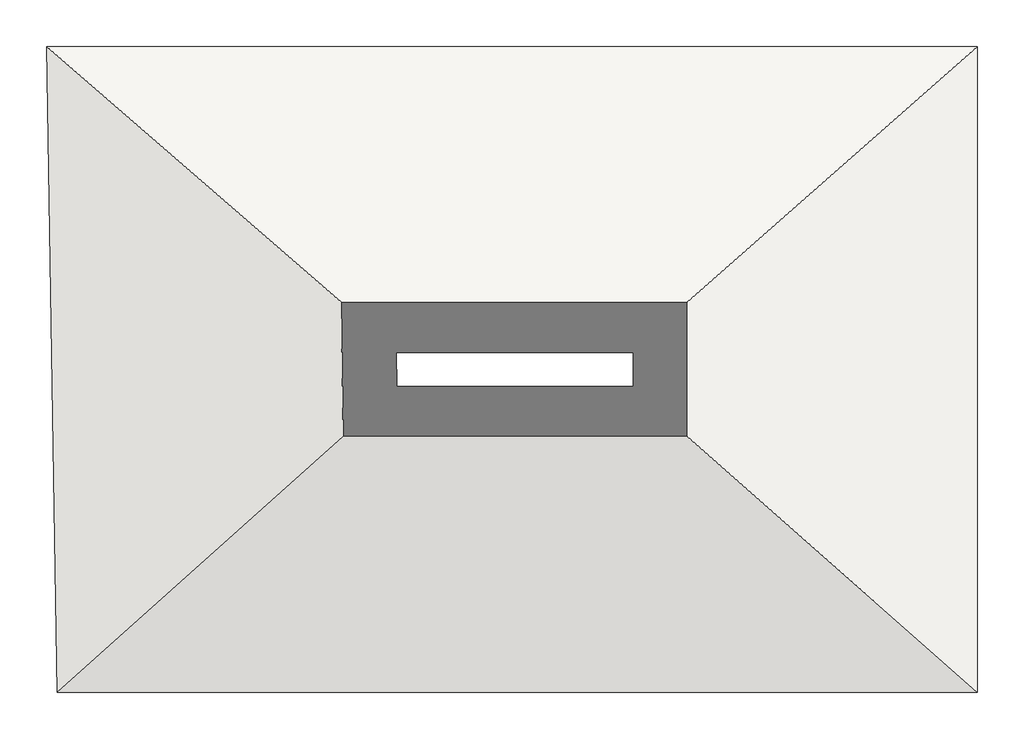
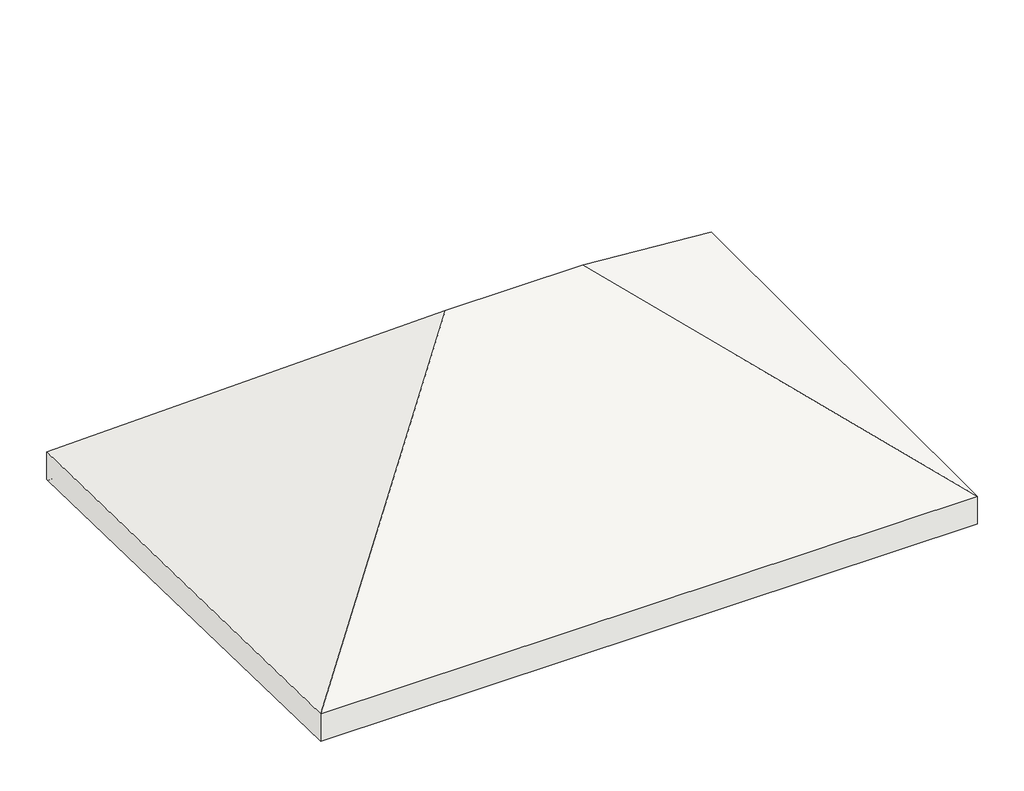
# One storey: 1 roof.
"""IFC4 building model written with IfcOpenShell, lengths in millimetres."""

from ifc_helpers import new_model, si_unit, origin, place, context, project, spatial, faceted_brep, element, save

model = new_model("IFC4")

# Units and contexts
model_context = context("Model", 3, world=origin())
ifc_project = project(units=[si_unit("LENGTHUNIT", "METRE", prefix="MILLI")], contexts=[model_context])

# Site, building, storey
site = spatial("IfcSite", under=ifc_project)
building = spatial("IfcBuilding", under=site)
storey = spatial("IfcBuildingStorey", under=building, Elevation=8534.4)

# Roof
placement = place(None, origin())
element("IfcRoof", 1, ObjectType="roofing 6\"", at=placement, inside=storey, context=model_context, shape_type="Brep", body=[
    faceted_brep([(-2723.0718918, 5449.6118978, 8534.4), (-4410.4081812, 3962.295896, 9799.9022171), (-5328.093256, 3962.295896, 9799.9022171), (-7040.8806375, 5449.6118978, 8534.4), (-2723.0718918, 2474.9798943, 8534.4), (-6990.463146, 2474.9798943, 8534.4), (-2723.0718918, 5460.895896, 8724.9), (-7041.0718918, 5460.895896, 8724.9), (-5315.2899013, 3962.295896, 10000.0033542), (-4423.2096973, 3962.295896, 10000.0033542), (-2723.0718918, 2463.695896, 8724.9), (-6990.2718918, 2463.695896, 8724.9), (-7041.0718918, 5460.895896, 8534.4), (-2723.0718918, 5460.895896, 8534.4), (-6990.2718918, 2463.695896, 8534.4), (-2723.0718918, 2463.695896, 8534.4)], [[[0, 1, 2, 3]], [[1, 0, 4]], [[5, 2, 1, 4]], [[3, 2, 5]], [[6, 7, 8, 9]], [[6, 9, 10]], [[11, 10, 9, 8]], [[7, 11, 8]], [[12, 7, 6, 13]], [[14, 11, 7, 12, 3, 5]], [[15, 10, 11, 14]], [[13, 6, 10, 15, 4, 0]], [[13, 0, 3, 12]], [[4, 15, 14, 5]]]),
])

save(model, "model.ifc")

# Revit data of these elements
# Type "roofing 6\""
#   Assembly Code = "B1020"
#   Layers, outside or top first: 0' - 6" "ROOFING 1'" (function 1)
# Element 1 (IfcRoof, "roofing 6\"")
#   built-in parameter 1001705 = 32.8084 (stored number, unit not read)
#   built-in parameter 1001710 = 33615
#   Phase Created = New Construction
#   Materials on its faces: "ROOFING 1'"
# Materials
#   "ROOFING 1'": class "Generic", colour RGB 120 120 120, transparency 0, Cost = 0
